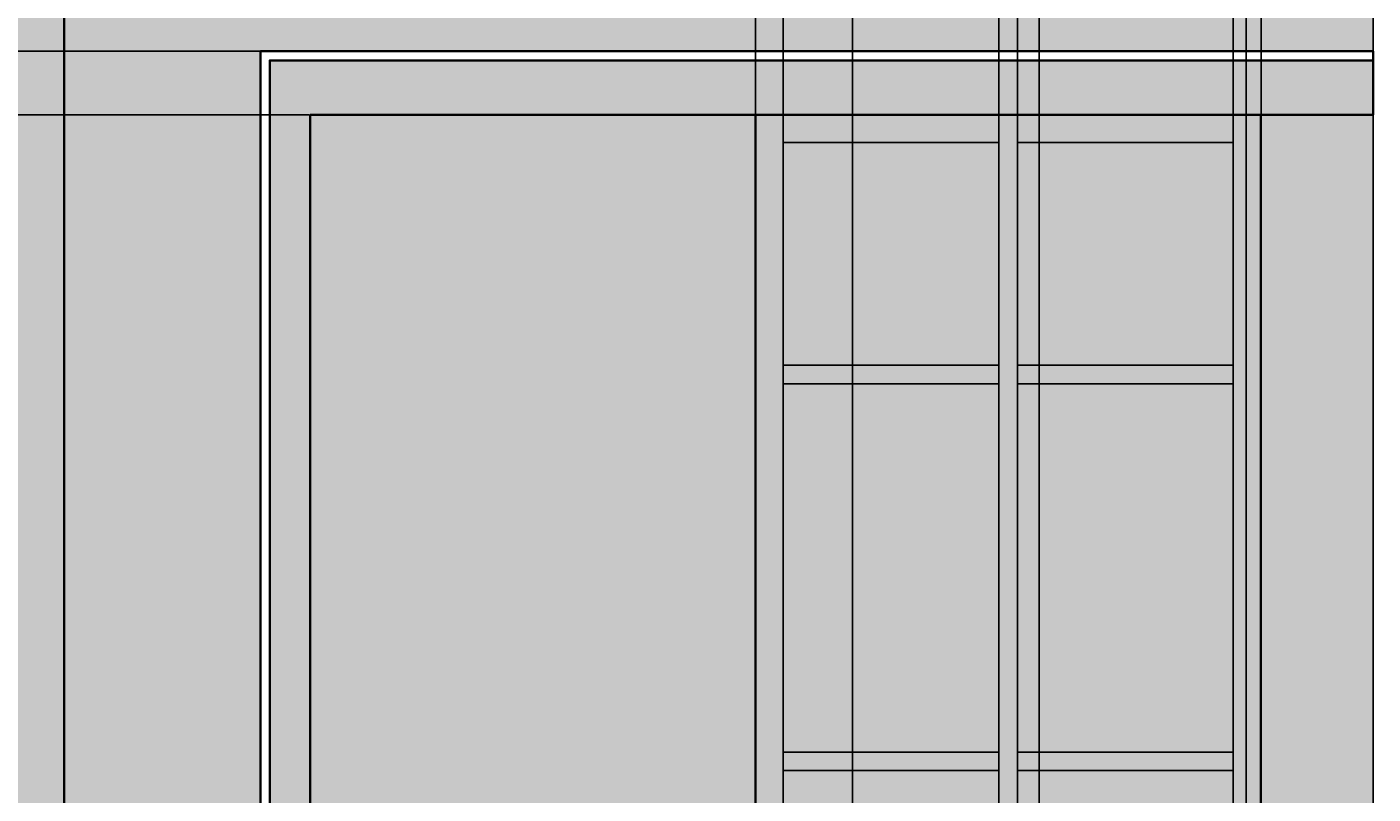
# Model space of a CAD drawing. Units: inches. Extents: x 62 to 566, y 66 to 528.
# Tile 8 of 20: x 138 to 284, y 347 to 430. Entities that reach past the tile are written whole.
import ezdxf

# ---------------------------------------------------------------- set-up
doc = ezdxf.new("R2010")
doc.units = ezdxf.units.IN
doc.header["$MEASUREMENT"] = 0
for name, color, linetype, lineweight in [('A-ANNO-DIMS', 2, 'Continuous', 18), ('A-ELEV', 7, 'Continuous', 35), ('A-GLAZ', 3, 'Continuous', 25), ('A-WALL-PATT', 8, 'Continuous', 13)]:
    doc.layers.add(name, color=color, linetype=linetype, lineweight=lineweight)
doc.styles.get("Standard").update_dxf_attribs({"font": 'arial.ttf'})
doc.dimstyles.get("Standard").update_dxf_attribs({"dimtxt": 0.75, "dimasz": 0.18, "dimexe": 0.18, "dimexo": 0.0625, "dimgap": 0.09, "dimtad": 0, "dimtih": 1, "dimtoh": 1, "dimdec": 4, "dimzin": 0, "dimdsep": 46, "dimlunit": 4, "dimtxsty": 'Standard', "dimcen": 0.09, "dimadec": 0, "dimazin": 0, "dimtfac": 1, "dimtdec": 4, "dimtofl": 0, "dimtmove": 0, "dimatfit": 3, "dimfxl": 1, "dimtolj": 1, "dimtzin": 0, "dimarcsym": 0})

# ---------------------------------------------------------------- blocks, each defined once
blk = doc.blocks.new('WIN-FRENCH-GRID')
for p, q in [((26.39, 108.06), (26.39, 83.9)), ((28.39, 108.06), (28.39, 83.9)), ((26.39, 83.9), (3, 83.9)), ((51.78, 83.9), (28.39, 83.9)), ((26.39, 81.9), (3, 81.9)), ((26.39, 81.9), (26.39, 41.97)), ((51.78, 81.9), (28.39, 81.9)), ((28.39, 81.9), (28.39, 41.97)), ((26.39, 41.97), (3, 41.97)), ((51.78, 41.97), (28.39, 41.97)), ((26.39, 39.97), (3, 39.97)), ((26.39, 39.97), (26.39, 3)), ((51.78, 39.97), (28.39, 39.97)), ((28.39, 39.97), (28.39, 3))]:
    blk.add_line(p, q)
blk.add_lwpolyline([(0, 111.06), (54.78, 111.06), (54.78, 0), (0, 0)], close=True)
for points in [[(3, 83.9), (3, 108.06), (26.39, 108.06)], [(28.39, 108.06), (51.78, 108.06), (51.78, 83.9)], [(3, 41.97), (3, 81.9)], [(51.78, 81.9), (51.78, 41.97)], [(26.39, 3), (3, 3), (3, 39.97)], [(51.78, 39.97), (51.78, 3), (28.39, 3)]]:
    blk.add_lwpolyline(points)
blk = doc.blocks.new('*D35')
at = {"layer": 'A-ANNO-DIMS', "color": 0, "lineweight": -2, "transparency": 16777216}
for p, q in [((125.94, 461.98), (125.94, 65.94)), ((142.39, 445.04), (142.39, 65.94)), ((126.12, 66.12), (132.55, 66.12)), ((142.21, 66.12), (135.77, 66.12))]:
    blk.add_line(p, q, dxfattribs=at)
at = {"layer": 'A-ANNO-DIMS', "color": 0, "transparency": 16777216}
for points in [[(126.12, 66.15), (126.12, 66.09), (125.94, 66.12)], [(142.21, 66.15), (142.21, 66.09), (142.39, 66.12)]]:
    blk.add_solid(points, dxfattribs=at)
at = {"layer": 'Defpoints', "color": 0, "transparency": 16777216}
for p in [(125.94, 462.04), (142.39, 445.11), (142.39, 66.12)]:
    blk.add_point(p, dxfattribs=at)
at = {"layer": 'A-ANNO-DIMS', "color": 0, "transparency": 16777216, "insert": (134.16, 66.12), "char_height": 0.75, "attachment_point": 5}
blk.add_mtext('\\A1;16.443', dxfattribs=at)
blk = doc.blocks.new('*D36')
at = {"layer": 'A-ANNO-DIMS', "color": 0, "lineweight": -2, "transparency": 16777216}
for p, q in [((142.39, 445.04), (142.39, 65.94)), ((163.65, 427.41), (163.65, 65.94)), ((142.57, 66.12), (151.66, 66.12)), ((163.47, 66.12), (154.38, 66.12))]:
    blk.add_line(p, q, dxfattribs=at)
at = {"layer": 'A-ANNO-DIMS', "color": 0, "transparency": 16777216}
for points in [[(142.57, 66.15), (142.57, 66.09), (142.39, 66.12)], [(163.47, 66.15), (163.47, 66.09), (163.65, 66.12)]]:
    blk.add_solid(points, dxfattribs=at)
at = {"layer": 'Defpoints', "color": 0, "transparency": 16777216}
for p in [(142.39, 445.11), (163.65, 427.48), (163.65, 66.12)]:
    blk.add_point(p, dxfattribs=at)
at = {"layer": 'A-ANNO-DIMS', "color": 0, "transparency": 16777216, "insert": (153.02, 66.12), "char_height": 0.75, "attachment_point": 5}
blk.add_mtext('\\A1;21.27', dxfattribs=at)
blk = doc.blocks.new('*D37')
at = {"layer": 'A-ANNO-DIMS', "color": 0, "lineweight": -2, "transparency": 16777216}
for p, q in [((163.65, 427.41), (163.65, 65.94)), ((169.04, 420.53), (169.04, 65.94)), ((163.83, 66.12), (164.99, 66.12)), ((168.86, 66.12), (167.71, 66.12))]:
    blk.add_line(p, q, dxfattribs=at)
at = {"layer": 'A-ANNO-DIMS', "color": 0, "transparency": 16777216}
for points in [[(163.83, 66.15), (163.83, 66.09), (163.65, 66.12)], [(168.86, 66.15), (168.86, 66.09), (169.04, 66.12)]]:
    blk.add_solid(points, dxfattribs=at)
at = {"layer": 'Defpoints', "color": 0, "transparency": 16777216}
for p in [(163.65, 427.48), (169.04, 420.6), (169.04, 66.12)]:
    blk.add_point(p, dxfattribs=at)
at = {"layer": 'A-ANNO-DIMS', "color": 0, "transparency": 16777216, "insert": (166.35, 66.12), "char_height": 0.75, "attachment_point": 5}
blk.add_mtext('\\A1;5.388', dxfattribs=at)
blk = doc.blocks.new('*D38')
at = {"layer": 'A-ANNO-DIMS', "color": 0, "lineweight": -2, "transparency": 16777216}
for p, q in [((169.04, 420.53), (169.04, 65.94)), ((217.28, 420.53), (217.28, 65.94)), ((169.22, 66.12), (191.79, 66.12)), ((217.1, 66.12), (194.53, 66.12))]:
    blk.add_line(p, q, dxfattribs=at)
at = {"layer": 'A-ANNO-DIMS', "color": 0, "transparency": 16777216}
for points in [[(169.22, 66.15), (169.22, 66.09), (169.04, 66.12)], [(217.1, 66.15), (217.1, 66.09), (217.28, 66.12)]]:
    blk.add_solid(points, dxfattribs=at)
at = {"layer": 'Defpoints', "color": 0, "transparency": 16777216}
for p in [(169.04, 420.6), (217.28, 420.6), (217.28, 66.12)]:
    blk.add_point(p, dxfattribs=at)
at = {"layer": 'A-ANNO-DIMS', "color": 0, "transparency": 16777216, "insert": (193.16, 66.12), "char_height": 0.75, "attachment_point": 5}
blk.add_mtext('\\A1;48.23', dxfattribs=at)
blk = doc.blocks.new('*D39')
at = {"layer": 'A-ANNO-DIMS', "color": 0, "lineweight": -2, "transparency": 16777216}
for p, q in [((284.2, 445.04), (284.2, 65.94)), ((217.28, 420.53), (217.28, 65.94)), ((217.46, 66.12), (249.38, 66.12)), ((284.02, 66.12), (252.1, 66.12))]:
    blk.add_line(p, q, dxfattribs=at)
at = {"layer": 'A-ANNO-DIMS', "color": 0, "transparency": 16777216}
for points in [[(217.46, 66.15), (217.46, 66.09), (217.28, 66.12)], [(284.02, 66.15), (284.02, 66.09), (284.2, 66.12)]]:
    blk.add_solid(points, dxfattribs=at)
at = {"layer": 'Defpoints', "color": 0, "transparency": 16777216}
for p in [(284.2, 445.11), (217.28, 420.6), (284.2, 66.12)]:
    blk.add_point(p, dxfattribs=at)
at = {"layer": 'A-ANNO-DIMS', "color": 0, "transparency": 16777216, "insert": (250.74, 66.12), "char_height": 0.75, "attachment_point": 5}
blk.add_mtext('\\A1;66.93', dxfattribs=at)
blk = doc.blocks.new('*D40')
at = {"layer": 'A-ANNO-DIMS', "color": 0, "lineweight": -2, "transparency": 16777216}
for p, q in [((284.2, 445.04), (284.2, 65.94)), ((316.21, 417.64), (316.21, 65.94)), ((284.38, 66.12), (298.92, 66.12)), ((316.03, 66.12), (301.49, 66.12))]:
    blk.add_line(p, q, dxfattribs=at)
at = {"layer": 'A-ANNO-DIMS', "color": 0, "transparency": 16777216}
for points in [[(284.38, 66.15), (284.38, 66.09), (284.2, 66.12)], [(316.03, 66.15), (316.03, 66.09), (316.21, 66.12)]]:
    blk.add_solid(points, dxfattribs=at)
at = {"layer": 'Defpoints', "color": 0, "transparency": 16777216}
for p in [(284.2, 445.11), (316.21, 417.71), (316.21, 66.12)]:
    blk.add_point(p, dxfattribs=at)
at = {"layer": 'A-ANNO-DIMS', "color": 0, "transparency": 16777216, "insert": (300.21, 66.12), "char_height": 0.75, "attachment_point": 5}
blk.add_mtext('\\A1;32.01', dxfattribs=at)
blk = doc.blocks.new('*D44')
at = {"layer": 'A-ANNO-DIMS', "color": 0, "lineweight": -2, "transparency": 16777216}
for p, q in [((163.59, 427.48), (63.47, 427.48)), ((63.65, 427.3), (63.65, 424.51)), ((63.65, 420.78), (63.65, 423.56)), ((168.98, 420.6), (63.47, 420.6))]:
    blk.add_line(p, q, dxfattribs=at)
at = {"layer": 'A-ANNO-DIMS', "color": 0, "transparency": 16777216}
for points in [[(63.62, 427.3), (63.68, 427.3), (63.65, 427.48)], [(63.62, 420.78), (63.68, 420.78), (63.65, 420.6)]]:
    blk.add_solid(points, dxfattribs=at)
at = {"layer": 'Defpoints', "color": 0, "transparency": 16777216}
for p in [(63.65, 427.48), (163.65, 427.48), (169.04, 420.6)]:
    blk.add_point(p, dxfattribs=at)
at = {"layer": 'A-ANNO-DIMS', "color": 0, "transparency": 16777216, "insert": (63.65, 424.04), "char_height": 0.75, "attachment_point": 5}
blk.add_mtext('\\A1;6.878', dxfattribs=at)
blk = doc.blocks.new('*D45')
at = {"layer": 'A-ANNO-DIMS', "color": 0, "lineweight": -2, "transparency": 16777216}
for p, q in [((142.32, 445.11), (63.47, 445.11)), ((63.65, 444.93), (63.65, 436.76)), ((63.65, 427.66), (63.65, 435.82)), ((163.59, 427.48), (63.47, 427.48))]:
    blk.add_line(p, q, dxfattribs=at)
at = {"layer": 'A-ANNO-DIMS', "color": 0, "transparency": 16777216}
for points in [[(63.62, 444.93), (63.68, 444.93), (63.65, 445.11)], [(63.62, 427.66), (63.68, 427.66), (63.65, 427.48)]]:
    blk.add_solid(points, dxfattribs=at)
at = {"layer": 'Defpoints', "color": 0, "transparency": 16777216}
for p in [(63.65, 445.11), (142.39, 445.11), (163.65, 427.48)]:
    blk.add_point(p, dxfattribs=at)
at = {"layer": 'A-ANNO-DIMS', "color": 0, "transparency": 16777216, "insert": (63.65, 436.29), "char_height": 0.75, "attachment_point": 5}
blk.add_mtext('\\A1;17.63', dxfattribs=at)
blk = doc.blocks.new('*D74')
at = {"layer": 'A-ANNO-DIMS', "color": 0, "lineweight": -2, "transparency": 16777216}
for p, q in [((284.2, 342.84), (284.2, 527.47)), ((284.38, 527.29), (292.86, 527.29)), ((304.64, 527.29), (296.16, 527.29)), ((304.82, 342.84), (304.82, 527.47))]:
    blk.add_line(p, q, dxfattribs=at)
at = {"layer": 'A-ANNO-DIMS', "color": 0, "transparency": 16777216}
for points in [[(284.38, 527.32), (284.38, 527.26), (284.2, 527.29)], [(304.64, 527.32), (304.64, 527.26), (304.82, 527.29)]]:
    blk.add_solid(points, dxfattribs=at)
at = {"layer": 'Defpoints', "color": 0, "transparency": 16777216}
for p in [(304.82, 527.29), (284.2, 342.78), (304.82, 342.78)]:
    blk.add_point(p, dxfattribs=at)
at = {"layer": 'A-ANNO-DIMS', "color": 0, "transparency": 16777216, "insert": (294.51, 527.29), "char_height": 0.75, "attachment_point": 5}
blk.add_mtext('\\A1;20.614', dxfattribs=at)
blk = doc.blocks.new('*D104')
at = {"layer": 'A-ANNO-DIMS', "color": 0, "lineweight": -2, "transparency": 16777216}
for p, q in [((217.28, 271.48), (217.28, 527.47)), ((217.46, 527.29), (218.44, 527.29)), ((220.1, 527.29), (219.11, 527.29)), ((220.28, 268.48), (220.28, 527.47))]:
    blk.add_line(p, q, dxfattribs=at)
at = {"layer": 'A-ANNO-DIMS', "color": 0, "transparency": 16777216}
for points in [[(217.46, 527.32), (217.46, 527.26), (217.28, 527.29)], [(220.1, 527.32), (220.1, 527.26), (220.28, 527.29)]]:
    blk.add_solid(points, dxfattribs=at)
at = {"layer": 'Defpoints', "color": 0, "transparency": 16777216}
for p in [(220.28, 527.29), (217.28, 271.41), (220.28, 268.41)]:
    blk.add_point(p, dxfattribs=at)
at = {"layer": 'A-ANNO-DIMS', "color": 0, "transparency": 16777216, "insert": (218.78, 527.29), "char_height": 0.75, "attachment_point": 5}
blk.add_mtext('\\A1;3', dxfattribs=at)
blk = doc.blocks.new('*D105')
at = {"layer": 'A-ANNO-DIMS', "color": 0, "lineweight": -2, "transparency": 16777216}
for p, q in [((220.28, 268.48), (220.28, 527.47)), ((220.46, 527.29), (230.61, 527.29)), ((243.49, 527.29), (233.33, 527.29)), ((243.67, 268.48), (243.67, 527.47))]:
    blk.add_line(p, q, dxfattribs=at)
at = {"layer": 'A-ANNO-DIMS', "color": 0, "transparency": 16777216}
for points in [[(220.46, 527.32), (220.46, 527.26), (220.28, 527.29)], [(243.49, 527.32), (243.49, 527.26), (243.67, 527.29)]]:
    blk.add_solid(points, dxfattribs=at)
at = {"layer": 'Defpoints', "color": 0, "transparency": 16777216}
for p in [(243.67, 527.29), (220.28, 268.41), (243.67, 268.41)]:
    blk.add_point(p, dxfattribs=at)
at = {"layer": 'A-ANNO-DIMS', "color": 0, "transparency": 16777216, "insert": (231.97, 527.29), "char_height": 0.75, "attachment_point": 5}
blk.add_mtext('\\A1;23.39', dxfattribs=at)
blk = doc.blocks.new('*D106')
at = {"layer": 'A-ANNO-DIMS', "color": 0, "lineweight": -2, "transparency": 16777216}
for p, q in [((243.67, 268.48), (243.67, 527.47)), ((243.85, 527.29), (244.33, 527.29)), ((245.49, 527.29), (245.01, 527.29)), ((245.67, 268.48), (245.67, 527.47))]:
    blk.add_line(p, q, dxfattribs=at)
at = {"layer": 'A-ANNO-DIMS', "color": 0, "transparency": 16777216}
for points in [[(243.85, 527.32), (243.85, 527.26), (243.67, 527.29)], [(245.49, 527.32), (245.49, 527.26), (245.67, 527.29)]]:
    blk.add_solid(points, dxfattribs=at)
at = {"layer": 'Defpoints', "color": 0, "transparency": 16777216}
for p in [(245.67, 527.29), (243.67, 268.41), (245.67, 268.41)]:
    blk.add_point(p, dxfattribs=at)
at = {"layer": 'A-ANNO-DIMS', "color": 0, "transparency": 16777216, "insert": (244.67, 527.29), "char_height": 0.75, "attachment_point": 5}
blk.add_mtext('\\A1;2', dxfattribs=at)
blk = doc.blocks.new('*D107')
at = {"layer": 'A-ANNO-DIMS', "color": 0, "lineweight": -2, "transparency": 16777216}
for p, q in [((245.67, 268.48), (245.67, 527.47)), ((245.85, 527.29), (256, 527.29)), ((268.88, 527.29), (258.73, 527.29)), ((269.06, 268.48), (269.06, 527.47))]:
    blk.add_line(p, q, dxfattribs=at)
at = {"layer": 'A-ANNO-DIMS', "color": 0, "transparency": 16777216}
for points in [[(245.85, 527.32), (245.85, 527.26), (245.67, 527.29)], [(268.88, 527.32), (268.88, 527.26), (269.06, 527.29)]]:
    blk.add_solid(points, dxfattribs=at)
at = {"layer": 'Defpoints', "color": 0, "transparency": 16777216}
for p in [(269.06, 527.29), (245.67, 268.41), (269.06, 268.41)]:
    blk.add_point(p, dxfattribs=at)
at = {"layer": 'A-ANNO-DIMS', "color": 0, "transparency": 16777216, "insert": (257.36, 527.29), "char_height": 0.75, "attachment_point": 5}
blk.add_mtext('\\A1;23.39', dxfattribs=at)
blk = doc.blocks.new('*D108')
at = {"layer": 'A-ANNO-DIMS', "color": 0, "lineweight": -2, "transparency": 16777216}
for p, q in [((269.06, 268.48), (269.06, 527.47)), ((269.24, 527.29), (270.22, 527.29)), ((271.88, 527.29), (270.89, 527.29)), ((272.06, 271.48), (272.06, 527.47))]:
    blk.add_line(p, q, dxfattribs=at)
at = {"layer": 'A-ANNO-DIMS', "color": 0, "transparency": 16777216}
for points in [[(269.24, 527.32), (269.24, 527.26), (269.06, 527.29)], [(271.88, 527.32), (271.88, 527.26), (272.06, 527.29)]]:
    blk.add_solid(points, dxfattribs=at)
at = {"layer": 'Defpoints', "color": 0, "transparency": 16777216}
for p in [(272.06, 527.29), (272.06, 271.41), (269.06, 268.41)]:
    blk.add_point(p, dxfattribs=at)
at = {"layer": 'A-ANNO-DIMS', "color": 0, "transparency": 16777216, "insert": (270.56, 527.29), "char_height": 0.75, "attachment_point": 5}
blk.add_mtext('\\A1;3', dxfattribs=at)
blk = doc.blocks.new('*D109')
at = {"layer": 'A-ANNO-DIMS', "color": 0, "lineweight": -2, "transparency": 16777216}
for p, q in [((217.28, 307.48), (217.28, 527.47)), ((217.46, 527.29), (220.92, 527.29)), ((227.62, 527.29), (224.15, 527.29)), ((227.8, 297.23), (227.8, 527.47))]:
    blk.add_line(p, q, dxfattribs=at)
at = {"layer": 'A-ANNO-DIMS', "color": 0, "transparency": 16777216}
for points in [[(217.46, 527.32), (217.46, 527.26), (217.28, 527.29)], [(227.62, 527.32), (227.62, 527.26), (227.8, 527.29)]]:
    blk.add_solid(points, dxfattribs=at)
at = {"layer": 'Defpoints', "color": 0, "transparency": 16777216}
for p in [(227.8, 527.29), (217.28, 307.41), (227.8, 297.17)]:
    blk.add_point(p, dxfattribs=at)
at = {"layer": 'A-ANNO-DIMS', "color": 0, "transparency": 16777216, "insert": (222.54, 527.29), "char_height": 0.75, "attachment_point": 5}
blk.add_mtext('\\A1;10.525', dxfattribs=at)
blk = doc.blocks.new('*D110')
at = {"layer": 'A-ANNO-DIMS', "color": 0, "lineweight": -2, "transparency": 16777216}
for p, q in [((227.8, 297.23), (227.8, 527.47)), ((227.98, 527.29), (236.26, 527.29)), ((247.83, 527.29), (239.56, 527.29)), ((248.01, 297.23), (248.01, 527.47))]:
    blk.add_line(p, q, dxfattribs=at)
at = {"layer": 'A-ANNO-DIMS', "color": 0, "transparency": 16777216}
for points in [[(227.98, 527.32), (227.98, 527.26), (227.8, 527.29)], [(247.83, 527.32), (247.83, 527.26), (248.01, 527.29)]]:
    blk.add_solid(points, dxfattribs=at)
at = {"layer": 'Defpoints', "color": 0, "transparency": 16777216}
for p in [(248.01, 527.29), (227.8, 297.17), (248.01, 297.17)]:
    blk.add_point(p, dxfattribs=at)
at = {"layer": 'A-ANNO-DIMS', "color": 0, "transparency": 16777216, "insert": (237.91, 527.29), "char_height": 0.75, "attachment_point": 5}
blk.add_mtext('\\A1;20.214', dxfattribs=at)
blk = doc.blocks.new('*D111')
at = {"layer": 'A-ANNO-DIMS', "color": 0, "lineweight": -2, "transparency": 16777216}
for p, q in [((248.01, 297.23), (248.01, 527.47)), ((248.19, 527.29), (257.87, 527.29)), ((270.26, 527.29), (260.59, 527.29)), ((270.44, 297.23), (270.44, 527.47))]:
    blk.add_line(p, q, dxfattribs=at)
at = {"layer": 'A-ANNO-DIMS', "color": 0, "transparency": 16777216}
for points in [[(248.19, 527.32), (248.19, 527.26), (248.01, 527.29)], [(270.26, 527.32), (270.26, 527.26), (270.44, 527.29)]]:
    blk.add_solid(points, dxfattribs=at)
at = {"layer": 'Defpoints', "color": 0, "transparency": 16777216}
for p in [(270.44, 527.29), (248.01, 297.17), (270.44, 297.17)]:
    blk.add_point(p, dxfattribs=at)
at = {"layer": 'A-ANNO-DIMS', "color": 0, "transparency": 16777216, "insert": (259.23, 527.29), "char_height": 0.75, "attachment_point": 5}
blk.add_mtext('\\A1;22.43', dxfattribs=at)
blk = doc.blocks.new('*D112')
at = {"layer": 'A-ANNO-DIMS', "color": 0, "lineweight": -2, "transparency": 16777216}
for p, q in [((270.44, 297.23), (270.44, 527.47)), ((270.62, 527.29), (276, 527.29)), ((284.02, 527.29), (278.64, 527.29)), ((284.2, 307.48), (284.2, 527.47))]:
    blk.add_line(p, q, dxfattribs=at)
at = {"layer": 'A-ANNO-DIMS', "color": 0, "transparency": 16777216}
for points in [[(270.62, 527.32), (270.62, 527.26), (270.44, 527.29)], [(284.02, 527.32), (284.02, 527.26), (284.2, 527.29)]]:
    blk.add_solid(points, dxfattribs=at)
at = {"layer": 'Defpoints', "color": 0, "transparency": 16777216}
for p in [(284.2, 527.29), (284.2, 307.41), (270.44, 297.17)]:
    blk.add_point(p, dxfattribs=at)
at = {"layer": 'A-ANNO-DIMS', "color": 0, "transparency": 16777216, "insert": (277.32, 527.29), "char_height": 0.75, "attachment_point": 5}
blk.add_mtext('\\A1;13.76', dxfattribs=at)

msp = doc.modelspace()

# ---------------------------------------------------------------- hatches: boundary and pattern name
at = {"layer": 'A-WALL-PATT'}
h = msp.add_hatch(color=256, dxfattribs=at)
h.dxf.hatch_style = 1
h.paths.add_polyline_path([(416.0836, 462.0423), (125.9418, 462.0423), (125.9418, 414.3686), (125.9418, 270.3686), (125.9418, 126.3686), (142.3851, 126.3686), (142.3851, 270.3686), (142.3851, 414.3686), (142.3851, 445.1064), (284.2021, 445.1064), (416.0836, 445.1064)])
h.paths.add_polyline_path([(435.3945, 503.0423), (426.3652, 503.0423), (120.4058, 503.0423), (120.4058, 501.0423), (125.9418, 501.0423), (416.0836, 501.0423), (426.3652, 501.0423), (430.6938, 501.0423), (435.3945, 501.0423)])
h.paths.add_polyline_path([(439.6878, 352.4848), (392.4793, 352.4848), (392.4793, 307.4128), (217.2752, 307.4128), (217.2752, 295.4098), (217.2752, 271.4128), (272.0586, 271.4128), (439.6878, 271.4128)])
h.paths.add_polyline_path([(248.0143, 297.1682), (255.6783, 297.1682), (255.6783, 280.0423), (248.0143, 280.0423)], flags=16)
h.paths.add_polyline_path([(235.4641, 280.0423), (227.8001, 280.0423), (227.8001, 297.1682), (235.4641, 297.1682)], flags=16)
h.paths.add_polyline_path([(270.4427, 297.1682), (278.1067, 297.1682), (278.1067, 280.0423), (270.4427, 280.0423)], flags=16)
h.paths.add_polyline_path([(296.3755, 297.1682), (304.0395, 297.1682), (304.0395, 280.0423), (296.3755, 280.0423)], flags=16)
h.paths.add_polyline_path([(319.2543, 297.1682), (326.9183, 297.1682), (326.9183, 280.0423), (319.2543, 280.0423)], flags=16)
h.paths.add_polyline_path([(341.2622, 297.1682), (348.9262, 297.1682), (348.9262, 280.0423), (341.2622, 280.0423)], flags=16)
h.paths.add_polyline_path([(389.2857, 298.3985), (433.8102, 298.3985), (433.8102, 294.9497), (389.2857, 294.9497)], flags=16)
h.paths.add_polyline_path([(389.2857, 291.6038), (433.8102, 291.6038), (433.8102, 288.155), (389.2857, 288.155)], flags=16)
h.paths.add_polyline_path([(389.2857, 284.9607), (433.8102, 284.9607), (433.8102, 281.5119), (389.2857, 281.5119)], flags=16)
h.paths.add_polyline_path([(403.5849, 311.4736), (403.5849, 317.4388), (433.1636, 317.4388), (433.1636, 311.4736)], flags=16)
h.paths.add_polyline_path([(403.5849, 323.1329), (403.5849, 329.0982), (433.1636, 329.0982), (433.1636, 323.1329)], flags=16)
h.paths.add_polyline_path([(403.5849, 334.5211), (403.5849, 340.4863), (433.1636, 340.4863), (433.1636, 334.5211)], flags=16)
h.paths.add_polyline_path([(272.0586, 160.3545), (217.2752, 160.3545), (217.2752, 129.0504), (217.2752, 126.3686), (272.0586, 126.3686)], flags=17)
h.paths.add_polyline_path([(220.5897, 149.5749), (220.5897, 152.296), (267.7931, 152.296), (267.7931, 149.5749)], flags=16)
h.paths.add_polyline_path([(267.7931, 146.6724), (267.7931, 143.9513), (220.5897, 143.9513), (220.5897, 146.6724)], flags=16)
h.paths.add_polyline_path([(220.5897, 155.3799), (220.5897, 158.101), (267.7931, 158.101), (267.7931, 155.3799)], flags=16)
h.paths.add_polyline_path([(267.7931, 140.686), (267.7931, 137.9649), (220.5897, 137.9649), (220.5897, 140.686)], flags=16)
h.paths.add_polyline_path([(267.7931, 135.516), (267.7931, 132.7949), (220.5897, 132.7949), (220.5897, 135.516)], flags=16)
h = msp.add_hatch(dxfattribs=at)
h.set_pattern_fill('ANSI36', color=256, scale=8.8)
h.paths.add_polyline_path([(217.2752, 420.597), (169.0431, 420.597), (169.0431, 126.3686), (217.2752, 126.3686), (217.2752, 129.0504), (217.2752, 271.4128), (217.2752, 295.4128), (217.2752, 307.4128)])
h.paths.add_polyline_path([(282.3509, 501.0423), (125.9418, 501.0423), (125.9418, 465.0423), (282.3509, 465.0423)])
h.paths.add_polyline_path([(209.709, 476.6506), (202.045, 476.6506), (202.045, 493.7764), (209.709, 493.7764)], flags=16)
h.paths.add_polyline_path([(193.9913, 476.6506), (186.3273, 476.6506), (186.3273, 493.7764), (193.9913, 493.7764)], flags=16)
h.paths.add_polyline_path([(177.9243, 476.6506), (170.2603, 476.6506), (170.2603, 493.7764), (177.9243, 493.7764)], flags=16)
h.paths.add_polyline_path([(163.2545, 476.3015), (155.5905, 476.3015), (155.5905, 493.4274), (163.2545, 493.4274)], flags=16)
h.paths.add_polyline_path([(148.2354, 476.3015), (140.5713, 476.3015), (140.5713, 493.4274), (148.2354, 493.4274)], flags=16)
h.paths.add_polyline_path([(284.2021, 126.3686), (87.8962, 126.3686), (87.8962, 114.3686), (87.8962, 90.3686), (284.2021, 90.3686)])
h.paths.add_polyline_path([(474.1214, 126.3686), (396.433, 126.3686), (396.433, 90.3686), (474.1214, 90.3686)])
h = msp.add_hatch(color=256, dxfattribs=at)
h.dxf.hatch_style = 1
h.paths.add_polyline_path([(416.0836, 501.0423), (282.3509, 501.0423), (282.3509, 465.0423), (416.0836, 465.0423)])
h.paths.add_polyline_path([(284.2021, 420.597), (272.0586, 420.597), (272.0586, 309.5388), (272.0586, 307.4128), (284.2021, 307.4128)], flags=17)
h.paths.add_polyline_path([(284.2021, 445.1064), (142.3851, 445.1064), (142.3851, 414.3686), (142.3851, 270.3686), (142.3851, 126.3686), (163.6548, 126.3686), (163.6548, 270.5016), (163.6548, 414.5016), (163.6548, 427.4752), (284.2021, 427.4752)])
h.paths.add_polyline_path([(235.4641, 297.1682), (227.8001, 297.1682), (227.8001, 280.0423), (235.4641, 280.0423)], flags=17)
h.paths.add_polyline_path([(255.6783, 297.1682), (248.0143, 297.1682), (248.0143, 280.0423), (255.6783, 280.0423)], flags=17)
h.paths.add_polyline_path([(278.1067, 297.1682), (270.4427, 297.1682), (270.4427, 280.0423), (278.1067, 280.0423)], flags=17)
h.paths.add_polyline_path([(304.0395, 297.1682), (296.3755, 297.1682), (296.3755, 280.0423), (304.0395, 280.0423)])
h.paths.add_polyline_path([(326.9183, 297.1682), (319.2543, 297.1682), (319.2543, 280.0423), (326.9183, 280.0423)])
h.paths.add_polyline_path([(348.9262, 297.1682), (341.2622, 297.1682), (341.2622, 280.0423), (348.9262, 280.0423)])
h.paths.add_polyline_path([(433.8102, 284.9607), (389.2857, 284.9607), (389.2857, 281.5119), (433.8102, 281.5119)])
h.paths.add_polyline_path([(433.8102, 291.6038), (389.2857, 291.6038), (389.2857, 288.155), (433.8102, 288.155)])
h.paths.add_polyline_path([(433.8102, 298.3985), (389.2857, 298.3985), (389.2857, 294.9497), (433.8102, 294.9497)])
h.paths.add_polyline_path([(433.1636, 317.4388), (403.5849, 317.4388), (403.5849, 311.4736), (433.1636, 311.4736)])
h.paths.add_polyline_path([(433.1636, 329.0982), (403.5849, 329.0982), (403.5849, 323.1329), (433.1636, 323.1329)])
h.paths.add_polyline_path([(433.1636, 340.4863), (403.5849, 340.4863), (403.5849, 334.5211), (433.1636, 334.5211)])
h.paths.add_polyline_path([(284.2021, 271.4128), (272.0586, 271.4128), (272.0586, 160.3545), (272.0586, 126.3686), (284.2021, 126.3686)])
h.paths.add_polyline_path([(267.7931, 158.101), (220.5897, 158.101), (220.5897, 155.3799), (267.7931, 155.3799)], flags=17)
h.paths.add_polyline_path([(267.7931, 152.296), (220.5897, 152.296), (220.5897, 149.5749), (267.7931, 149.5749)], flags=17)
h.paths.add_polyline_path([(267.7931, 146.6724), (220.5897, 146.6724), (220.5897, 143.9513), (267.7931, 143.9513)], flags=17)
h.paths.add_polyline_path([(267.7931, 140.686), (220.5897, 140.686), (220.5897, 137.9649), (267.7931, 137.9649)], flags=17)
h.paths.add_polyline_path([(267.7931, 135.516), (220.5897, 135.516), (220.5897, 132.7949), (267.7931, 132.7949)], flags=17)
h.paths.add_polyline_path([(148.2354, 493.4274), (140.5713, 493.4274), (140.5713, 476.3015), (148.2354, 476.3015)])
h.paths.add_polyline_path([(163.2545, 493.4274), (155.5905, 493.4274), (155.5905, 476.3015), (163.2545, 476.3015)])
h.paths.add_polyline_path([(177.9243, 493.7764), (170.2603, 493.7764), (170.2603, 476.6506), (177.9243, 476.6506)])
h.paths.add_polyline_path([(193.9913, 493.7764), (186.3273, 493.7764), (186.3273, 476.6506), (193.9913, 476.6506)])
h.paths.add_polyline_path([(209.709, 493.7764), (202.045, 493.7764), (202.045, 476.6506), (209.709, 476.6506)])
h = msp.add_hatch(color=256, dxfattribs=at)
h.dxf.hatch_style = 1
h.paths.add_polyline_path([(430.6938, 462.0423), (416.0836, 462.0423), (416.0836, 445.1064), (430.6938, 445.1064)])
h.paths.add_polyline_path([(169.0431, 420.597), (284.2021, 420.597), (284.2021, 426.4752), (164.6548, 426.4752), (164.6548, 414.5016), (164.6548, 126.3686), (169.0431, 126.3686)])
h = msp.add_hatch(color=256, dxfattribs=at)
h.dxf.hatch_style = 1
h.paths.add_polyline_path([(272.0586, 420.597), (217.2752, 420.597), (217.2752, 309.5388), (272.0586, 309.5388)])
h.paths.add_polyline_path([(245.6669, 393.435), (245.6669, 417.597), (269.0586, 417.597), (269.0586, 393.435)], flags=16)
h.paths.add_polyline_path([(245.6669, 391.435), (269.0586, 391.435), (269.0586, 351.5079), (245.6669, 351.5079)], flags=16)
h.paths.add_polyline_path([(243.6669, 393.435), (220.2752, 393.435), (220.2752, 417.597), (243.6669, 417.597)], flags=16)
h.paths.add_polyline_path([(243.6669, 391.435), (243.6669, 351.5079), (220.2752, 351.5079), (220.2752, 391.435)], flags=16)
h.paths.add_polyline_path([(245.6669, 349.5079), (269.0586, 349.5079), (269.0586, 312.5388), (245.6669, 312.5388)], flags=16)
h.paths.add_polyline_path([(243.6669, 349.5079), (243.6669, 312.5388), (220.2752, 312.5388), (220.2752, 349.5079)], flags=16)
h.paths.add_polyline_path([(272.0586, 271.4128), (217.2752, 271.4128), (217.2752, 160.3545), (272.0586, 160.3545)])
h.paths.add_polyline_path([(243.6669, 268.4128), (243.6669, 244.2507), (220.2752, 244.2507), (220.2752, 268.4128)], flags=16)
h.paths.add_polyline_path([(245.6669, 268.4128), (269.0586, 268.4128), (269.0586, 244.2507), (245.6669, 244.2507)], flags=16)
h.paths.add_polyline_path([(243.6669, 242.2507), (243.6669, 202.3236), (220.2752, 202.3236), (220.2752, 242.2507)], flags=16)
h.paths.add_polyline_path([(245.6669, 242.2507), (269.0586, 242.2507), (269.0586, 202.3236), (245.6669, 202.3236)], flags=16)
h.paths.add_polyline_path([(243.6669, 200.3236), (243.6669, 163.3545), (220.2752, 163.3545), (220.2752, 200.3236)], flags=16)
h.paths.add_polyline_path([(245.6669, 200.3236), (269.0586, 200.3236), (269.0586, 163.3545), (245.6669, 163.3545)], flags=16)
h.paths.add_polyline_path([(272.0586, 309.5388), (217.2752, 309.5388), (217.2752, 307.4128), (272.0586, 307.4128)])
h = msp.add_hatch(color=256, dxfattribs=at)
h.dxf.hatch_style = 1
h.set_gradient(color1=(0, 0, 255), color2=(0, 0, 0))
h.paths.add_polyline_path([(243.6669, 417.597), (220.2752, 417.597), (220.2752, 393.435), (243.6669, 393.435)])
h.paths.add_polyline_path([(269.0586, 417.597), (245.6669, 417.597), (245.6669, 393.435), (269.0586, 393.435)])
h.paths.add_polyline_path([(269.0586, 391.435), (245.6669, 391.435), (245.6669, 351.5079), (269.0586, 351.5079)])
h.paths.add_polyline_path([(243.6669, 391.435), (220.2752, 391.435), (220.2752, 351.5079), (243.6669, 351.5079)])
h.paths.add_polyline_path([(243.6669, 349.5079), (220.2752, 349.5079), (220.2752, 312.5388), (243.6669, 312.5388)])
h.paths.add_polyline_path([(269.0586, 349.5079), (245.6669, 349.5079), (245.6669, 312.5388), (269.0586, 312.5388)])
h.paths.add_polyline_path([(243.6669, 268.4128), (220.2752, 268.4128), (220.2752, 244.2507), (243.6669, 244.2507)])
h.paths.add_polyline_path([(269.0586, 268.4128), (245.6669, 268.4128), (245.6669, 244.2507), (269.0586, 244.2507)])
h.paths.add_polyline_path([(269.0586, 242.2507), (245.6669, 242.2507), (245.6669, 202.3236), (269.0586, 202.3236)])
h.paths.add_polyline_path([(243.6669, 242.2507), (220.2752, 242.2507), (220.2752, 202.3236), (243.6669, 202.3236)])
h.paths.add_polyline_path([(243.6669, 200.3236), (220.2752, 200.3236), (220.2752, 163.3545), (243.6669, 163.3545)])
h.paths.add_polyline_path([(269.0586, 200.3236), (245.6669, 200.3236), (245.6669, 163.3545), (269.0586, 163.3545)])
h = msp.add_hatch(color=256, dxfattribs=at)
h.dxf.hatch_style = 1
h.paths.add_polyline_path([(245.6669, 417.597), (243.6669, 417.597), (243.6669, 393.435), (220.2752, 393.435), (220.2752, 391.435), (243.6669, 391.435), (243.6669, 351.5079), (220.2752, 351.5079), (220.2752, 349.5079), (243.6669, 349.5079), (243.6669, 312.5388), (245.6669, 312.5388), (245.6669, 349.5079), (269.0586, 349.5079), (269.0586, 351.5079), (245.6669, 351.5079), (245.6669, 391.435), (269.0586, 391.435), (269.0586, 393.435), (245.6669, 393.435)], flags=0)

# ---------------------------------------------------------------- linework, layer by layer
at = {"layer": 'A-ELEV'}
for p, q in [((142.3851, 414.3686), (142.3851, 445.1064)), ((169.0431, 126.3686), (169.0431, 420.597)), ((217.2752, 307.4128), (217.2752, 420.597)), ((272.0586, 309.5388), (272.0586, 420.597)), ((142.3851, 270.3686), (142.3851, 414.3686))]:
    msp.add_line(p, q, dxfattribs=at)
for points in [[(163.6548, 126.3686), (163.6548, 414.5016), (163.6548, 427.4752), (284.2021, 427.4752)], [(169.0431, 420.597), (284.2021, 420.597), (284.2021, 427.4752)], [(164.6548, 126.3686), (164.6548, 414.5016), (164.6548, 426.4752), (284.2021, 426.4752)]]:
    msp.add_lwpolyline(points, dxfattribs=at)

# ---------------------------------------------------------------- block references
at = {"layer": 'A-GLAZ'}
msp.add_blockref('WIN-FRENCH-GRID', (217.2752, 309.5388), dxfattribs=at)

# ---------------------------------------------------------------- dimensions: what is measured, and where the dimension line sits
at = {"layer": 'A-ANNO-DIMS'}
for base, p1, p2, override, picture, middle in [((220.2752, 527.2923), (217.2752, 271.4128), (220.2752, 268.4128), {"dimdec": 0, "dimlfac": 1, "dimrnd": 0, "dimzin": 0, "dimdsep": 46, "dimlunit": 2}, '*D104', (218.7752, 527.2923)), ((227.8001, 527.2923), (217.2752, 307.4128), (227.8001, 297.1682), {"dimdec": 3, "dimlfac": 1, "dimrnd": 0, "dimzin": 0, "dimdsep": 46, "dimlunit": 2}, '*D109', (222.5377, 527.2923)), ((243.6669, 527.2923), (220.2752, 268.4128), (243.6669, 268.4128), {"dimdec": 2, "dimlfac": 1, "dimrnd": 0, "dimzin": 0, "dimdsep": 46, "dimlunit": 2}, '*D105', (231.971, 527.2923)), ((248.0143, 527.2923), (227.8001, 297.1682), (248.0143, 297.1682), {"dimdec": 3, "dimlfac": 1, "dimrnd": 0, "dimzin": 0, "dimdsep": 46, "dimlunit": 2}, '*D110', (237.9072, 527.2923)), ((245.6669, 527.2923), (243.6669, 268.4128), (245.6669, 268.4128), {"dimdec": 0, "dimlfac": 1, "dimrnd": 0, "dimzin": 0, "dimdsep": 46, "dimlunit": 2}, '*D106', (244.6669, 527.2923)), ((269.0586, 527.2923), (245.6669, 268.4128), (269.0586, 268.4128), {"dimdec": 2, "dimlfac": 1, "dimrnd": 0, "dimzin": 0, "dimdsep": 46, "dimlunit": 2}, '*D107', (257.3627, 527.2923)), ((270.4427, 527.2923), (248.0143, 297.1682), (270.4427, 297.1682), {"dimdec": 2, "dimlfac": 1, "dimrnd": 0, "dimzin": 0, "dimdsep": 46, "dimlunit": 2}, '*D111', (259.2285, 527.2923)), ((272.0586, 527.2923), (269.0586, 268.4128), (272.0586, 271.4128), {"dimdec": 0, "dimlfac": 1, "dimrnd": 0, "dimzin": 0, "dimdsep": 46, "dimlunit": 2}, '*D108', (270.5586, 527.2923)), ((284.2021, 527.2923), (270.4427, 297.1682), (284.2021, 307.4128), {"dimdec": 2, "dimlfac": 1, "dimrnd": 0, "dimzin": 0, "dimdsep": 46, "dimlunit": 2}, '*D112', (277.3224, 527.2923)), ((304.8163, 527.2923), (284.2021, 342.7821), (304.8163, 342.7821), {"dimdec": 3, "dimlfac": 1, "dimrnd": 0, "dimzin": 0, "dimdsep": 46, "dimlunit": 2}, '*D74', (294.5092, 527.2923)), ((142.3851, 66.1186), (125.9418, 462.0423), (142.3851, 445.1064), {"dimdec": 3, "dimlfac": 1, "dimrnd": 0, "dimzin": 0, "dimdsep": 46, "dimlunit": 2}, '*D35', (134.1634, 66.1186)), ((163.6548, 66.1186), (142.3851, 445.1064), (163.6548, 427.4752), {"dimdec": 2, "dimlfac": 1, "dimrnd": 0, "dimzin": 0, "dimdsep": 46, "dimlunit": 2}, '*D36', (153.0199, 66.1186)), ((284.2021, 66.1186), (217.2752, 420.597), (284.2021, 445.1064), {"dimdec": 2, "dimlfac": 1, "dimrnd": 0, "dimzin": 0, "dimdsep": 46, "dimlunit": 2}, '*D39', (250.7386, 66.1186)), ((316.2101, 66.1186), (284.2021, 445.1064), (316.2101, 417.7059), {"dimdec": 2, "dimlfac": 1, "dimrnd": 0, "dimzin": 0, "dimdsep": 46, "dimlunit": 2}, '*D40', (300.2061, 66.1186)), ((169.0431, 66.1186), (163.6548, 427.4752), (169.0431, 420.597), {"dimdec": 3, "dimlfac": 1, "dimrnd": 0, "dimzin": 0, "dimdsep": 46, "dimlunit": 2}, '*D37', (166.349, 66.1186)), ((217.2752, 66.1186), (169.0431, 420.597), (217.2752, 420.597), {"dimdec": 2, "dimlfac": 1, "dimrnd": 0, "dimzin": 0, "dimdsep": 46, "dimlunit": 2}, '*D38', (193.1592, 66.1186))]:
    dim = msp.add_linear_dim(base=base, p1=p1, p2=p2, dimstyle='Standard', override=override, dxfattribs=at)
    dim.commit()
    dim.dimension.update_dxf_attribs({"geometry": picture, "text_midpoint": middle})
for base, p1, p2, override, picture, middle in [((63.6462, 445.1064), (163.6548, 427.4752), (142.3851, 445.1064), {"dimdec": 2, "dimlfac": 1, "dimrnd": 0, "dimzin": 0, "dimdsep": 46, "dimlunit": 2}, '*D45', (63.6462, 436.2908)), ((63.6462, 427.4752), (169.0431, 420.597), (163.6548, 427.4752), {"dimdec": 3, "dimlfac": 1, "dimrnd": 0, "dimzin": 0, "dimdsep": 46, "dimlunit": 2}, '*D44', (63.6462, 424.0361))]:
    dim = msp.add_linear_dim(base=base, p1=p1, p2=p2, angle=90, dimstyle='Standard', override=override, dxfattribs=at)
    dim.commit()
    dim.dimension.update_dxf_attribs({"geometry": picture, "text_midpoint": middle})

doc.saveas('drawing.dxf')
